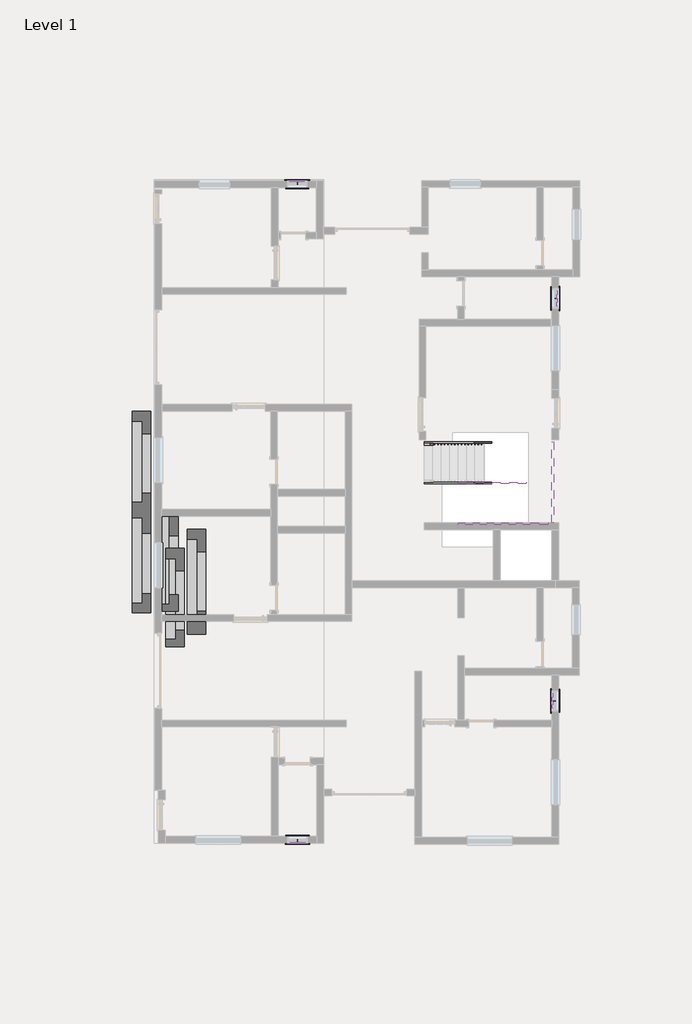
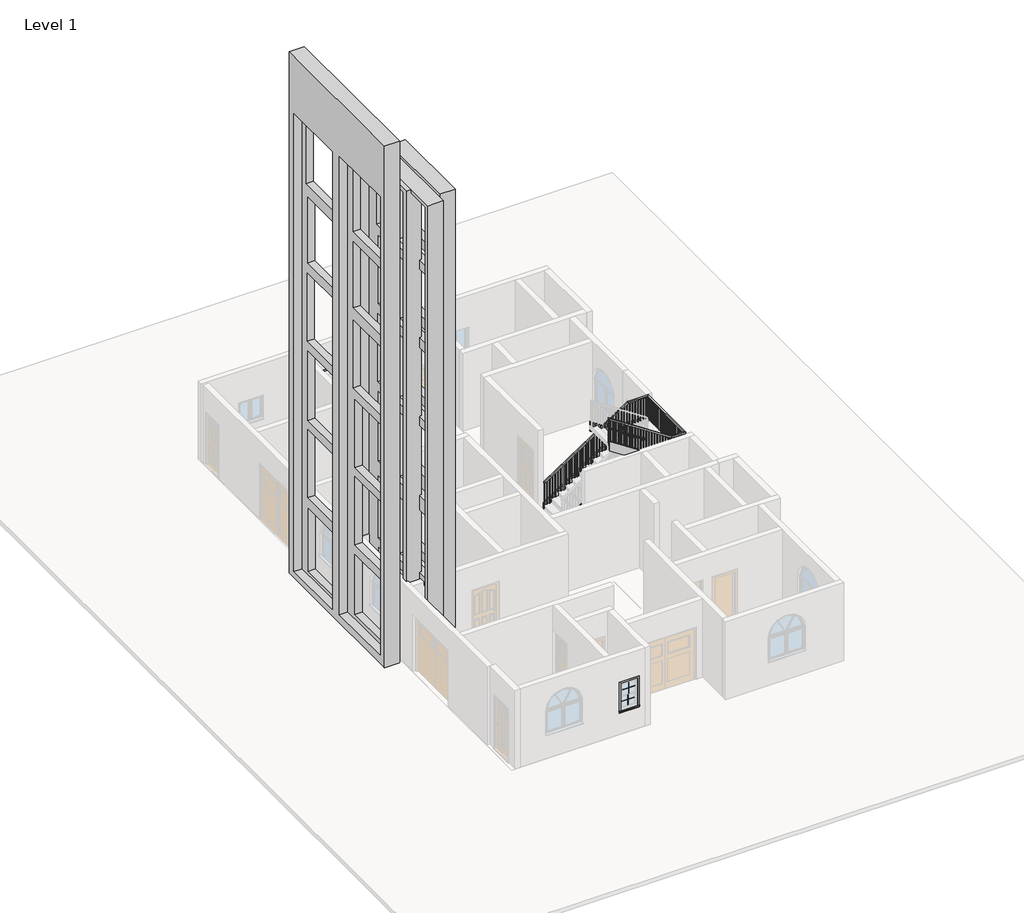
# One storey, part 4 of 4: 20 proxies, 5 members, 1 railing.
"""IFC4 building model written with IfcOpenShell, lengths in millimetres."""

from ifc_helpers import new_model, si_unit, frame, origin, place, context, project, spatial, polyline, outline, extrude, faceted_brep, transform, mapped, element, save
from components import generic_models_1_generic_models_1_14763b5c, generic_models_2_generic_models_1_16343201, generic_models_3_generic_models_1_639dc579, generic_models_4_generic_models_1_30fca322, muntin_pattern_2x2_muntin_pattern_2x2_eba6c5fb, trim_window_exterior_flat_with_sill_278e6a94, trim_window_interior_flat_picture_frame_e9fd5f45

model = new_model("IFC4")

# Units and contexts
model_context = context("Model", 3, world=origin())
ifc_project = project(units=[si_unit("LENGTHUNIT", "METRE", prefix="MILLI")], contexts=[model_context])

# Site, building, storey
site = spatial("IfcSite", under=ifc_project)
building = spatial("IfcBuilding", under=site)
storey = spatial("IfcBuildingStorey", under=building, Name="Level 1", Elevation=0.0)

# Proxies
placement = place(None, origin())
generic_models_1_generic_models_1_shape = generic_models_1_generic_models_1_14763b5c(model_context)
element("IfcBuildingElementProxy", 1, Name="Generic Models 1 : Generic Models 1", ObjectType="Generic Models 1 : Generic Models 1", at=placement, inside=storey, context=model_context, shape_type="MappedRepresentation", body=[
    mapped(generic_models_1_generic_models_1_shape, transform((0.0, 0.0, 0.0), x_axis=(1.0, 0.0, 0.0), y_axis=(0.0, 1.0, 0.0), z_axis=(0.0, 0.0, 1.0))),
])
generic_models_2_generic_models_1_shape = generic_models_2_generic_models_1_16343201(model_context)
element("IfcBuildingElementProxy", 2, Name="Generic Models 2 : Generic Models 1", ObjectType="Generic Models 2 : Generic Models 1", at=placement, inside=storey, context=model_context, shape_type="MappedRepresentation", body=[
    mapped(generic_models_2_generic_models_1_shape, transform((824.2499329, -3076.1426277, 0.0), x_axis=(1.0, 0.0, 0.0), y_axis=(0.0, 1.0, 0.0), z_axis=(0.0, 0.0, 1.0))),
])
generic_models_3_generic_models_1_shape = generic_models_3_generic_models_1_639dc579(model_context)
element("IfcBuildingElementProxy", 3, Name="Generic Models 3 : Generic Models 1", ObjectType="Generic Models 3 : Generic Models 1", at=placement, inside=storey, context=model_context, shape_type="MappedRepresentation", body=[
    mapped(generic_models_3_generic_models_1_shape, transform((1011.525957, -4144.962921, 0.0), x_axis=(1.0, 0.0, 0.0), y_axis=(0.0, 1.0, 0.0), z_axis=(0.0, 0.0, 1.0))),
])
generic_models_4_generic_models_1_shape = generic_models_4_generic_models_1_30fca322(model_context)
element("IfcBuildingElementProxy", 4, Name="Generic Models 4 : Generic Models 1", ObjectType="Generic Models 4 : Generic Models 1", at=placement, inside=storey, context=model_context, shape_type="MappedRepresentation", body=[
    mapped(generic_models_4_generic_models_1_shape, transform((1663.8480965, -3568.1337576, 0.0), x_axis=(1.0, 0.0, 0.0), y_axis=(0.0, 1.0, 0.0), z_axis=(0.0, 0.0, 1.0))),
])
muntin_pattern_2x2_muntin_pattern_2x2_shape = muntin_pattern_2x2_muntin_pattern_2x2_eba6c5fb(model_context)
element("IfcBuildingElementProxy", 5, Name="Muntin Pattern_2x2 : Muntin Pattern_2x2", ObjectType="Muntin Pattern_2x2 : Muntin Pattern_2x2", at=placement, inside=storey, context=model_context, shape_type="MappedRepresentation", body=[
    mapped(muntin_pattern_2x2_muntin_pattern_2x2_shape, transform((5828.2640963, 5846.2962251, 1470.025), x_axis=(0.0, -1.0, 0.0), y_axis=(1.0, 0.0, 0.0), z_axis=(0.0, 0.0, 1.0))),
])
element("IfcBuildingElementProxy", 6, Name="Muntin Pattern_2x2 : Muntin Pattern_2x2", ObjectType="Muntin Pattern_2x2 : Muntin Pattern_2x2", at=placement, inside=storey, context=model_context, shape_type="MappedRepresentation", body=[
    mapped(muntin_pattern_2x2_muntin_pattern_2x2_shape, transform((5783.8140963, 5846.2962251, 990.6), x_axis=(0.0, -1.0, 0.0), y_axis=(1.0, 0.0, 0.0), z_axis=(0.0, 0.0, 1.0))),
])
element("IfcBuildingElementProxy", 7, Name="Muntin Pattern_2x2 : Muntin Pattern_2x2", ObjectType="Muntin Pattern_2x2 : Muntin Pattern_2x2", at=placement, inside=storey, context=model_context, shape_type="MappedRepresentation", body=[
    mapped(muntin_pattern_2x2_muntin_pattern_2x2_shape, transform((5694.9140963, -6313.9537749, 1470.025), x_axis=(0.0, 1.0, 0.0), y_axis=(-1.0, 0.0, 0.0), z_axis=(0.0, 0.0, 1.0))),
])
element("IfcBuildingElementProxy", 8, Name="Muntin Pattern_2x2 : Muntin Pattern_2x2", ObjectType="Muntin Pattern_2x2 : Muntin Pattern_2x2", at=placement, inside=storey, context=model_context, shape_type="MappedRepresentation", body=[
    mapped(muntin_pattern_2x2_muntin_pattern_2x2_shape, transform((5739.3640963, -6313.9537749, 990.6), x_axis=(0.0, 1.0, 0.0), y_axis=(-1.0, 0.0, 0.0), z_axis=(0.0, 0.0, 1.0))),
])
element("IfcBuildingElementProxy", 9, Name="Muntin Pattern_2x2 : Muntin Pattern_2x2", ObjectType="Muntin Pattern_2x2 : Muntin Pattern_2x2", at=placement, inside=storey, context=model_context, shape_type="MappedRepresentation", body=[
    mapped(muntin_pattern_2x2_muntin_pattern_2x2_shape, transform((-2029.8609037, 9366.9277313, 1470.025), x_axis=(1.0, 0.0, 0.0), y_axis=(0.0, 1.0, 0.0), z_axis=(0.0, 0.0, 1.0))),
])
element("IfcBuildingElementProxy", 10, Name="Muntin Pattern_2x2 : Muntin Pattern_2x2", ObjectType="Muntin Pattern_2x2 : Muntin Pattern_2x2", at=placement, inside=storey, context=model_context, shape_type="MappedRepresentation", body=[
    mapped(muntin_pattern_2x2_muntin_pattern_2x2_shape, transform((-2029.8609037, 9322.4777313, 990.6), x_axis=(1.0, 0.0, 0.0), y_axis=(0.0, 1.0, 0.0), z_axis=(0.0, 0.0, 1.0))),
])
element("IfcBuildingElementProxy", 11, Name="Muntin Pattern_2x2 : Muntin Pattern_2x2", ObjectType="Muntin Pattern_2x2 : Muntin Pattern_2x2", at=placement, inside=storey, context=model_context, shape_type="MappedRepresentation", body=[
    mapped(muntin_pattern_2x2_muntin_pattern_2x2_shape, transform((-2023.5109037, -10577.9787749, 1470.025), x_axis=(-1.0, 0.0, 0.0), y_axis=(0.0, -1.0, 0.0), z_axis=(0.0, 0.0, 1.0))),
])
element("IfcBuildingElementProxy", 12, Name="Muntin Pattern_2x2 : Muntin Pattern_2x2", ObjectType="Muntin Pattern_2x2 : Muntin Pattern_2x2", at=placement, inside=storey, context=model_context, shape_type="MappedRepresentation", body=[
    mapped(muntin_pattern_2x2_muntin_pattern_2x2_shape, transform((-2023.5109037, -10533.5287749, 990.6), x_axis=(-1.0, 0.0, 0.0), y_axis=(0.0, -1.0, 0.0), z_axis=(0.0, 0.0, 1.0))),
])
trim_window_exterior_flat_with_sill_shape = trim_window_exterior_flat_with_sill_278e6a94(model_context)
element("IfcBuildingElementProxy", 13, Name="Trim-Window-Exterior-Flat : with Sill", ObjectType="Trim-Window-Exterior-Flat : with Sill", at=placement, inside=storey, context=model_context, shape_type="MappedRepresentation", body=[
    mapped(trim_window_exterior_flat_with_sill_shape, transform((5863.1890963, 5846.2962251, 1981.2), x_axis=(0.0, 1.0, 0.0), y_axis=(0.0, 0.0, 1.0), z_axis=(1.0, 0.0, 0.0))),
])
element("IfcBuildingElementProxy", 14, Name="Trim-Window-Exterior-Flat : with Sill", ObjectType="Trim-Window-Exterior-Flat : with Sill", at=placement, inside=storey, context=model_context, shape_type="MappedRepresentation", body=[
    mapped(trim_window_exterior_flat_with_sill_shape, transform((5659.9890963, -6313.9537749, 1981.2), x_axis=(0.0, -1.0, 0.0), y_axis=(0.0, 0.0, 1.0), z_axis=(-1.0, 0.0, 0.0))),
])
element("IfcBuildingElementProxy", 15, Name="Trim-Window-Exterior-Flat : with Sill", ObjectType="Trim-Window-Exterior-Flat : with Sill", at=placement, inside=storey, context=model_context, shape_type="MappedRepresentation", body=[
    mapped(trim_window_exterior_flat_with_sill_shape, transform((-2029.8609037, 9401.8527313, 1981.2), x_axis=(-1.0, 0.0, 0.0), y_axis=(0.0, 0.0, 1.0), z_axis=(0.0, 1.0, 0.0))),
])
element("IfcBuildingElementProxy", 16, Name="Trim-Window-Exterior-Flat : with Sill", ObjectType="Trim-Window-Exterior-Flat : with Sill", at=placement, inside=storey, context=model_context, shape_type="MappedRepresentation", body=[
    mapped(trim_window_exterior_flat_with_sill_shape, transform((-2023.5109037, -10612.9037749, 1981.2), x_axis=(1.0, 0.0, 0.0), y_axis=(0.0, 0.0, 1.0), z_axis=(0.0, -1.0, 0.0))),
])
trim_window_interior_flat_picture_frame_shape = trim_window_interior_flat_picture_frame_e9fd5f45(model_context)
element("IfcBuildingElementProxy", 17, Name="Trim-Window-Interior-Flat : Picture Frame", ObjectType="Trim-Window-Interior-Flat : Picture Frame", at=placement, inside=storey, context=model_context, shape_type="MappedRepresentation", body=[
    mapped(trim_window_interior_flat_picture_frame_shape, transform((5659.9890963, 5846.2962251, 1981.2), x_axis=(0.0, -1.0, 0.0), y_axis=(0.0, 0.0, 1.0), z_axis=(-1.0, 0.0, 0.0))),
])
element("IfcBuildingElementProxy", 18, Name="Trim-Window-Interior-Flat : Picture Frame", ObjectType="Trim-Window-Interior-Flat : Picture Frame", at=placement, inside=storey, context=model_context, shape_type="MappedRepresentation", body=[
    mapped(trim_window_interior_flat_picture_frame_shape, transform((5863.1890963, -6313.9537749, 1981.2), x_axis=(0.0, 1.0, 0.0), y_axis=(0.0, 0.0, 1.0), z_axis=(1.0, 0.0, 0.0))),
])
element("IfcBuildingElementProxy", 19, Name="Trim-Window-Interior-Flat : Picture Frame", ObjectType="Trim-Window-Interior-Flat : Picture Frame", at=placement, inside=storey, context=model_context, shape_type="MappedRepresentation", body=[
    mapped(trim_window_interior_flat_picture_frame_shape, transform((-2029.8609037, 9198.6527313, 1981.2), x_axis=(1.0, 0.0, 0.0), y_axis=(0.0, 0.0, 1.0), z_axis=(0.0, -1.0, 0.0))),
])
element("IfcBuildingElementProxy", 20, Name="Trim-Window-Interior-Flat : Picture Frame", ObjectType="Trim-Window-Interior-Flat : Picture Frame", at=placement, inside=storey, context=model_context, shape_type="MappedRepresentation", body=[
    mapped(trim_window_interior_flat_picture_frame_shape, transform((-2023.5109037, -10409.7037749, 1981.2), x_axis=(-1.0, 0.0, 0.0), y_axis=(0.0, 0.0, 1.0), z_axis=(0.0, 1.0, 0.0))),
])

# Members
element("IfcMember", 21, ObjectType="Stringer - 2\" Width", at=placement, inside=storey, context=model_context, shape_type="SweptSolid", body=[
    extrude(outline(polyline([(218.8021702, 1811.8890963), (0.0, 1811.8890963), (0.0, 2033.570289), (2277.5333333, 5475.7230993), (2277.5333333, 4923.3549769), (218.8021702, 1811.8890963)])), frame((0.0, 1464.7962251, 0.0), z_axis=(0.0, 1.0, 0.0), x_axis=(0.0, 0.0, 1.0)), (0.0, 0.0, 1.0), 50.8),
])
element("IfcMember", 22, ObjectType="Stringer - 2\" Width", at=placement, inside=storey, context=model_context, shape_type="SweptSolid", body=[
    extrude(outline(polyline([(5659.9890963, 1515.5962251), (5710.7890963, 1515.5962251), (5710.7890963, -935.5037749), (5659.9890963, -935.5037749), (5659.9890963, 1515.5962251)])), frame((0.0, 0.0, 1972.7333333), z_axis=(0.0, 0.0, 1.0), x_axis=(1.0, 0.0, 0.0)), (0.0, 0.0, 1.0), 304.8),
])
element("IfcMember", 23, ObjectType="Stringer - 2\" Width", at=placement, inside=storey, context=model_context, shape_type="SweptSolid", body=[
    extrude(outline(polyline([(1972.7333333, 5557.7517847), (3771.2542006, 2827.8890963), (3406.2494122, 2827.8890963), (1972.7333333, 5003.7337741), (1972.7333333, 5557.7517847)])), frame((0.0, -986.3037749, 0.0), z_axis=(0.0, 1.0, 0.0), x_axis=(0.0, 0.0, 1.0)), (0.0, 0.0, 1.0), 50.8),
])
element("IfcMember", 24, ObjectType="Stringer - 2\" Width", at=placement, inside=storey, context=model_context, shape_type="SweptSolid", body=[
    extrude(outline(polyline([(218.8021702, 1811.8890963), (0.0, 1811.8890963), (0.0, 2033.570289), (1850.4384087, 4830.2326586), (2215.9180606, 4830.2326586), (218.8021702, 1811.8890963)])), frame((0.0, 245.5962251, 0.0), z_axis=(0.0, 1.0, 0.0), x_axis=(0.0, 0.0, 1.0)), (0.0, 0.0, 1.0), 50.8),
])
element("IfcMember", 25, ObjectType="Stringer - 2\" Width", at=placement, inside=storey, context=model_context, shape_type="SweptSolid", body=[
    extrude(outline(polyline([(2053.5727534, 4881.0326586), (2418.5775418, 4881.0326586), (3771.2542006, 2827.8890963), (3406.2494122, 2827.8890963), (2053.5727534, 4881.0326586)])), frame((0.0, 245.5962251, 0.0), z_axis=(0.0, 1.0, 0.0), x_axis=(0.0, 0.0, 1.0)), (0.0, 0.0, 1.0), 50.8),
])

# Railing
element("IfcRailing", 26, ObjectType="Handrail - Rectangular", at=placement, inside=storey, context=model_context, shape_type="SolidModel", body=[
    faceted_brep([(1811.8890963, 1464.7962251, 1083.7333333), (1811.8890963, 1464.7962251, 1022.8084396), (1811.8890963, 1413.9962251, 1022.8084396), (1811.8890963, 1413.9962251, 1083.7333333), (4881.0326586, 1464.7962251, 3115.7333333), (4896.3253517, 1464.7962251, 3064.9333333), (4896.3253517, 1413.9962251, 3064.9333333), (4881.0326586, 1413.9962251, 3115.7333333), (5659.9890963, 1464.7962251, 3115.7333333), (5659.9890963, 1464.7962251, 3064.9333333), (5609.1890963, 1413.9962251, 3064.9333333), (5609.1890963, 1413.9962251, 3115.7333333), (5659.9890963, -935.5037749, 3115.7333333), (5659.9890963, -935.5037749, 3064.9333333), (5609.1890963, -884.7037749, 3064.9333333), (5609.1890963, -884.7037749, 3115.7333333), (5137.6756039, -935.5037749, 3115.7333333), (5122.4267175, -935.5037749, 3064.9333333), (5122.4267175, -884.7037749, 3064.9333333), (5137.6756039, -884.7037749, 3115.7333333), (2827.8890963, -935.5037749, 4639.7333333), (2827.8890963, -884.7037749, 4639.7333333), (2827.8890963, -884.7037749, 4578.8720992), (2827.8890963, -935.5037749, 4578.8720992)], [[[0, 1, 2, 3]], [[1, 0, 4, 5]], [[2, 1, 5, 6]], [[3, 2, 6, 7]], [[0, 3, 7, 4]], [[5, 4, 8, 9]], [[6, 5, 9, 10]], [[7, 6, 10, 11]], [[4, 7, 11, 8]], [[9, 8, 12, 13]], [[10, 9, 13, 14]], [[11, 10, 14, 15]], [[8, 11, 15, 12]], [[13, 12, 16, 17]], [[14, 13, 17, 18]], [[15, 14, 18, 19]], [[12, 15, 19, 16]], [[20, 21, 22, 23]], [[17, 16, 20, 23]], [[18, 17, 23, 22]], [[19, 18, 22, 21]], [[16, 19, 21, 20]]]),
    extrude(outline(polyline([(4543.3154863, 2881.8640963), (3556.0, 2881.8640963), (3556.0, 2900.9140963), (4530.7029775, 2900.9140963), (4543.3154863, 2881.8640963)])), frame((0.0, -919.6287749, 0.0), z_axis=(0.0, 1.0, 0.0), x_axis=(0.0, 0.0, 1.0)), (0.0, 0.0, 1.0), 19.05),
    extrude(outline(polyline([(4476.2235214, 2983.4640963), (3556.0, 2983.4640963), (3556.0, 3002.5140963), (4463.6543078, 3002.5140963), (4476.2235214, 2983.4640963)])), frame((0.0, -919.6287749, 0.0), z_axis=(0.0, 1.0, 0.0), x_axis=(0.0, 0.0, 1.0)), (0.0, 0.0, 1.0), 19.05),
    extrude(outline(polyline([(4409.1877155, 3085.0640963), (3386.6666667, 3085.0640963), (3386.6666667, 3104.1140963), (4396.6185019, 3104.1140963), (4409.1877155, 3085.0640963)])), frame((0.0, -919.6287749, 0.0), z_axis=(0.0, 1.0, 0.0), x_axis=(0.0, 0.0, 1.0)), (0.0, 0.0, 1.0), 19.05),
    extrude(outline(polyline([(4342.1519096, 3186.6640963), (3386.6666667, 3186.6640963), (3386.6666667, 3205.7140963), (4329.582696, 3205.7140963), (4342.1519096, 3186.6640963)])), frame((0.0, -919.6287749, 0.0), z_axis=(0.0, 1.0, 0.0), x_axis=(0.0, 0.0, 1.0)), (0.0, 0.0, 1.0), 19.05),
    extrude(outline(polyline([(4275.1161037, 3288.2640963), (3386.6666667, 3288.2640963), (3386.6666667, 3307.3140963), (4262.5468901, 3307.3140963), (4275.1161037, 3288.2640963)])), frame((0.0, -919.6287749, 0.0), z_axis=(0.0, 1.0, 0.0), x_axis=(0.0, 0.0, 1.0)), (0.0, 0.0, 1.0), 19.05),
    extrude(outline(polyline([(4208.0802978, 3389.8640963), (3217.3333333, 3389.8640963), (3217.3333333, 3408.9140963), (4195.5110842, 3408.9140963), (4208.0802978, 3389.8640963)])), frame((0.0, -919.6287749, 0.0), z_axis=(0.0, 1.0, 0.0), x_axis=(0.0, 0.0, 1.0)), (0.0, 0.0, 1.0), 19.05),
    extrude(outline(polyline([(4141.0444919, 3491.4640963), (3217.3333333, 3491.4640963), (3217.3333333, 3510.5140963), (4128.4752783, 3510.5140963), (4141.0444919, 3491.4640963)])), frame((0.0, -919.6287749, 0.0), z_axis=(0.0, 1.0, 0.0), x_axis=(0.0, 0.0, 1.0)), (0.0, 0.0, 1.0), 19.05),
    extrude(outline(polyline([(4074.008686, 3593.0640963), (3048.0, 3593.0640963), (3048.0, 3612.1140963), (4061.4394724, 3612.1140963), (4074.008686, 3593.0640963)])), frame((0.0, -919.6287749, 0.0), z_axis=(0.0, 1.0, 0.0), x_axis=(0.0, 0.0, 1.0)), (0.0, 0.0, 1.0), 19.05),
    extrude(outline(polyline([(4006.9728801, 3694.6640963), (3048.0, 3694.6640963), (3048.0, 3713.7140963), (3994.4036665, 3713.7140963), (4006.9728801, 3694.6640963)])), frame((0.0, -919.6287749, 0.0), z_axis=(0.0, 1.0, 0.0), x_axis=(0.0, 0.0, 1.0)), (0.0, 0.0, 1.0), 19.05),
    extrude(outline(polyline([(3939.9370742, 3796.2640963), (3048.0, 3796.2640963), (3048.0, 3815.3140963), (3927.3678606, 3815.3140963), (3939.9370742, 3796.2640963)])), frame((0.0, -919.6287749, 0.0), z_axis=(0.0, 1.0, 0.0), x_axis=(0.0, 0.0, 1.0)), (0.0, 0.0, 1.0), 19.05),
    extrude(outline(polyline([(3872.9814538, 3897.8640963), (2878.6666667, 3897.8640963), (2878.6666667, 3916.9140963), (3860.3689451, 3916.9140963), (3872.9814538, 3897.8640963)])), frame((0.0, -919.6287749, 0.0), z_axis=(0.0, 1.0, 0.0), x_axis=(0.0, 0.0, 1.0)), (0.0, 0.0, 1.0), 19.05),
    extrude(outline(polyline([(3805.8654624, 3999.4640963), (2878.6666667, 3999.4640963), (2878.6666667, 4018.5140963), (3793.2962488, 4018.5140963), (3805.8654624, 3999.4640963)])), frame((0.0, -919.6287749, 0.0), z_axis=(0.0, 1.0, 0.0), x_axis=(0.0, 0.0, 1.0)), (0.0, 0.0, 1.0), 19.05),
    extrude(outline(polyline([(3738.8296565, 4101.0640963), (2709.3333333, 4101.0640963), (2709.3333333, 4120.1140963), (3726.2604429, 4120.1140963), (3738.8296565, 4101.0640963)])), frame((0.0, -919.6287749, 0.0), z_axis=(0.0, 1.0, 0.0), x_axis=(0.0, 0.0, 1.0)), (0.0, 0.0, 1.0), 19.05),
    extrude(outline(polyline([(3671.7938506, 4202.6640963), (2709.3333333, 4202.6640963), (2709.3333333, 4221.7140963), (3659.224637, 4221.7140963), (3671.7938506, 4202.6640963)])), frame((0.0, -919.6287749, 0.0), z_axis=(0.0, 1.0, 0.0), x_axis=(0.0, 0.0, 1.0)), (0.0, 0.0, 1.0), 19.05),
    extrude(outline(polyline([(3604.7580447, 4304.2640963), (2709.3333333, 4304.2640963), (2709.3333333, 4323.3140963), (3592.1888311, 4323.3140963), (3604.7580447, 4304.2640963)])), frame((0.0, -919.6287749, 0.0), z_axis=(0.0, 1.0, 0.0), x_axis=(0.0, 0.0, 1.0)), (0.0, 0.0, 1.0), 19.05),
    extrude(outline(polyline([(3537.7222388, 4405.8640963), (2540.0, 4405.8640963), (2540.0, 4424.9140963), (3525.1530252, 4424.9140963), (3537.7222388, 4405.8640963)])), frame((0.0, -919.6287749, 0.0), z_axis=(0.0, 1.0, 0.0), x_axis=(0.0, 0.0, 1.0)), (0.0, 0.0, 1.0), 19.05),
    extrude(outline(polyline([(3470.6864329, 4507.4640963), (2540.0, 4507.4640963), (2540.0, 4526.5140963), (3458.1172193, 4526.5140963), (3470.6864329, 4507.4640963)])), frame((0.0, -919.6287749, 0.0), z_axis=(0.0, 1.0, 0.0), x_axis=(0.0, 0.0, 1.0)), (0.0, 0.0, 1.0), 19.05),
    extrude(outline(polyline([(3403.650627, 4609.0640963), (2370.6666667, 4609.0640963), (2370.6666667, 4628.1140963), (3391.0814134, 4628.1140963), (3403.650627, 4609.0640963)])), frame((0.0, -919.6287749, 0.0), z_axis=(0.0, 1.0, 0.0), x_axis=(0.0, 0.0, 1.0)), (0.0, 0.0, 1.0), 19.05),
    extrude(outline(polyline([(3336.6148211, 4710.6640963), (2370.6666667, 4710.6640963), (2370.6666667, 4729.7140963), (3324.0456075, 4729.7140963), (3336.6148211, 4710.6640963)])), frame((0.0, -919.6287749, 0.0), z_axis=(0.0, 1.0, 0.0), x_axis=(0.0, 0.0, 1.0)), (0.0, 0.0, 1.0), 19.05),
    extrude(outline(polyline([(3269.5790152, 4812.2640963), (2370.6666667, 4812.2640963), (2370.6666667, 4831.3140963), (3257.0098016, 4831.3140963), (3269.5790152, 4812.2640963)])), frame((0.0, -919.6287749, 0.0), z_axis=(0.0, 1.0, 0.0), x_axis=(0.0, 0.0, 1.0)), (0.0, 0.0, 1.0), 19.05),
    extrude(outline(polyline([(3202.5432093, 4913.8640963), (2201.3333333, 4913.8640963), (2201.3333333, 4932.9140963), (3189.9739957, 4932.9140963), (3202.5432093, 4913.8640963)])), frame((0.0, -919.6287749, 0.0), z_axis=(0.0, 1.0, 0.0), x_axis=(0.0, 0.0, 1.0)), (0.0, 0.0, 1.0), 19.05),
    extrude(outline(polyline([(3135.5074034, 5015.4640963), (2201.3333333, 5015.4640963), (2201.3333333, 5034.5140963), (3122.9381898, 5034.5140963), (3135.5074034, 5015.4640963)])), frame((0.0, -919.6287749, 0.0), z_axis=(0.0, 1.0, 0.0), x_axis=(0.0, 0.0, 1.0)), (0.0, 0.0, 1.0), 19.05),
    extrude(outline(polyline([(3068.4715975, 5117.0640963), (2201.3333333, 5117.0640963), (2201.3333333, 5136.1140963), (3055.9023839, 5136.1140963), (3068.4715975, 5117.0640963)])), frame((0.0, -919.6287749, 0.0), z_axis=(0.0, 1.0, 0.0), x_axis=(0.0, 0.0, 1.0)), (0.0, 0.0, 1.0), 19.05),
    extrude(outline(polyline([(5237.7140963, -919.6287749), (5218.6640963, -919.6287749), (5218.6640963, -900.5787749), (5237.7140963, -900.5787749), (5237.7140963, -919.6287749)])), frame((0.0, 0.0, 2201.3333333), z_axis=(0.0, 0.0, 1.0), x_axis=(1.0, 0.0, 0.0)), (0.0, 0.0, 1.0), 863.6),
    extrude(outline(polyline([(5339.3140963, -919.6287749), (5320.2640963, -919.6287749), (5320.2640963, -900.5787749), (5339.3140963, -900.5787749), (5339.3140963, -919.6287749)])), frame((0.0, 0.0, 2201.3333333), z_axis=(0.0, 0.0, 1.0), x_axis=(1.0, 0.0, 0.0)), (0.0, 0.0, 1.0), 863.6),
    extrude(outline(polyline([(5440.9140963, -919.6287749), (5421.8640963, -919.6287749), (5421.8640963, -900.5787749), (5440.9140963, -900.5787749), (5440.9140963, -919.6287749)])), frame((0.0, 0.0, 2201.3333333), z_axis=(0.0, 0.0, 1.0), x_axis=(1.0, 0.0, 0.0)), (0.0, 0.0, 1.0), 863.6),
    extrude(outline(polyline([(5542.5140963, -919.6287749), (5523.4640963, -919.6287749), (5523.4640963, -900.5787749), (5542.5140963, -900.5787749), (5542.5140963, -919.6287749)])), frame((0.0, 0.0, 2201.3333333), z_axis=(0.0, 0.0, 1.0), x_axis=(1.0, 0.0, 0.0)), (0.0, 0.0, 1.0), 863.6),
    extrude(outline(polyline([(5644.1140963, -887.8787749), (5644.1140963, -906.9287749), (5625.0640963, -906.9287749), (5625.0640963, -887.8787749), (5644.1140963, -887.8787749)])), frame((0.0, 0.0, 2201.3333333), z_axis=(0.0, 0.0, 1.0), x_axis=(1.0, 0.0, 0.0)), (0.0, 0.0, 1.0), 863.6),
    extrude(outline(polyline([(5644.1140963, -786.2787749), (5644.1140963, -805.3287749), (5625.0640963, -805.3287749), (5625.0640963, -786.2787749), (5644.1140963, -786.2787749)])), frame((0.0, 0.0, 2201.3333333), z_axis=(0.0, 0.0, 1.0), x_axis=(1.0, 0.0, 0.0)), (0.0, 0.0, 1.0), 863.6),
    extrude(outline(polyline([(5644.1140963, -684.6787749), (5644.1140963, -703.7287749), (5625.0640963, -703.7287749), (5625.0640963, -684.6787749), (5644.1140963, -684.6787749)])), frame((0.0, 0.0, 2201.3333333), z_axis=(0.0, 0.0, 1.0), x_axis=(1.0, 0.0, 0.0)), (0.0, 0.0, 1.0), 863.6),
    extrude(outline(polyline([(5644.1140963, -583.0787749), (5644.1140963, -602.1287749), (5625.0640963, -602.1287749), (5625.0640963, -583.0787749), (5644.1140963, -583.0787749)])), frame((0.0, 0.0, 2201.3333333), z_axis=(0.0, 0.0, 1.0), x_axis=(1.0, 0.0, 0.0)), (0.0, 0.0, 1.0), 863.6),
    extrude(outline(polyline([(5644.1140963, -481.4787749), (5644.1140963, -500.5287749), (5625.0640963, -500.5287749), (5625.0640963, -481.4787749), (5644.1140963, -481.4787749)])), frame((0.0, 0.0, 2201.3333333), z_axis=(0.0, 0.0, 1.0), x_axis=(1.0, 0.0, 0.0)), (0.0, 0.0, 1.0), 863.6),
    extrude(outline(polyline([(5644.1140963, -379.8787749), (5644.1140963, -398.9287749), (5625.0640963, -398.9287749), (5625.0640963, -379.8787749), (5644.1140963, -379.8787749)])), frame((0.0, 0.0, 2201.3333333), z_axis=(0.0, 0.0, 1.0), x_axis=(1.0, 0.0, 0.0)), (0.0, 0.0, 1.0), 863.6),
    extrude(outline(polyline([(5644.1140963, -278.2787749), (5644.1140963, -297.3287749), (5625.0640963, -297.3287749), (5625.0640963, -278.2787749), (5644.1140963, -278.2787749)])), frame((0.0, 0.0, 2201.3333333), z_axis=(0.0, 0.0, 1.0), x_axis=(1.0, 0.0, 0.0)), (0.0, 0.0, 1.0), 863.6),
    extrude(outline(polyline([(5644.1140963, -176.6787749), (5644.1140963, -195.7287749), (5625.0640963, -195.7287749), (5625.0640963, -176.6787749), (5644.1140963, -176.6787749)])), frame((0.0, 0.0, 2201.3333333), z_axis=(0.0, 0.0, 1.0), x_axis=(1.0, 0.0, 0.0)), (0.0, 0.0, 1.0), 863.6),
    extrude(outline(polyline([(5644.1140963, -75.0787749), (5644.1140963, -94.1287749), (5625.0640963, -94.1287749), (5625.0640963, -75.0787749), (5644.1140963, -75.0787749)])), frame((0.0, 0.0, 2201.3333333), z_axis=(0.0, 0.0, 1.0), x_axis=(1.0, 0.0, 0.0)), (0.0, 0.0, 1.0), 863.6),
    extrude(outline(polyline([(5644.1140963, 26.5212251), (5644.1140963, 7.4712251), (5625.0640963, 7.4712251), (5625.0640963, 26.5212251), (5644.1140963, 26.5212251)])), frame((0.0, 0.0, 2201.3333333), z_axis=(0.0, 0.0, 1.0), x_axis=(1.0, 0.0, 0.0)), (0.0, 0.0, 1.0), 863.6),
    extrude(outline(polyline([(5644.1140963, 128.1212251), (5644.1140963, 109.0712251), (5625.0640963, 109.0712251), (5625.0640963, 128.1212251), (5644.1140963, 128.1212251)])), frame((0.0, 0.0, 2201.3333333), z_axis=(0.0, 0.0, 1.0), x_axis=(1.0, 0.0, 0.0)), (0.0, 0.0, 1.0), 863.6),
    extrude(outline(polyline([(5644.1140963, 229.7212251), (5644.1140963, 210.6712251), (5625.0640963, 210.6712251), (5625.0640963, 229.7212251), (5644.1140963, 229.7212251)])), frame((0.0, 0.0, 2201.3333333), z_axis=(0.0, 0.0, 1.0), x_axis=(1.0, 0.0, 0.0)), (0.0, 0.0, 1.0), 863.6),
    extrude(outline(polyline([(5644.1140963, 331.3212251), (5644.1140963, 312.2712251), (5625.0640963, 312.2712251), (5625.0640963, 331.3212251), (5644.1140963, 331.3212251)])), frame((0.0, 0.0, 2201.3333333), z_axis=(0.0, 0.0, 1.0), x_axis=(1.0, 0.0, 0.0)), (0.0, 0.0, 1.0), 863.6),
    extrude(outline(polyline([(5644.1140963, 432.9212251), (5644.1140963, 413.8712251), (5625.0640963, 413.8712251), (5625.0640963, 432.9212251), (5644.1140963, 432.9212251)])), frame((0.0, 0.0, 2201.3333333), z_axis=(0.0, 0.0, 1.0), x_axis=(1.0, 0.0, 0.0)), (0.0, 0.0, 1.0), 863.6),
    extrude(outline(polyline([(5644.1140963, 534.5212251), (5644.1140963, 515.4712251), (5625.0640963, 515.4712251), (5625.0640963, 534.5212251), (5644.1140963, 534.5212251)])), frame((0.0, 0.0, 2201.3333333), z_axis=(0.0, 0.0, 1.0), x_axis=(1.0, 0.0, 0.0)), (0.0, 0.0, 1.0), 863.6),
    extrude(outline(polyline([(5644.1140963, 636.1212251), (5644.1140963, 617.0712251), (5625.0640963, 617.0712251), (5625.0640963, 636.1212251), (5644.1140963, 636.1212251)])), frame((0.0, 0.0, 2201.3333333), z_axis=(0.0, 0.0, 1.0), x_axis=(1.0, 0.0, 0.0)), (0.0, 0.0, 1.0), 863.6),
    extrude(outline(polyline([(5644.1140963, 737.7212251), (5644.1140963, 718.6712251), (5625.0640963, 718.6712251), (5625.0640963, 737.7212251), (5644.1140963, 737.7212251)])), frame((0.0, 0.0, 2201.3333333), z_axis=(0.0, 0.0, 1.0), x_axis=(1.0, 0.0, 0.0)), (0.0, 0.0, 1.0), 863.6),
    extrude(outline(polyline([(5644.1140963, 839.3212251), (5644.1140963, 820.2712251), (5625.0640963, 820.2712251), (5625.0640963, 839.3212251), (5644.1140963, 839.3212251)])), frame((0.0, 0.0, 2201.3333333), z_axis=(0.0, 0.0, 1.0), x_axis=(1.0, 0.0, 0.0)), (0.0, 0.0, 1.0), 863.6),
    extrude(outline(polyline([(5644.1140963, 940.9212251), (5644.1140963, 921.8712251), (5625.0640963, 921.8712251), (5625.0640963, 940.9212251), (5644.1140963, 940.9212251)])), frame((0.0, 0.0, 2201.3333333), z_axis=(0.0, 0.0, 1.0), x_axis=(1.0, 0.0, 0.0)), (0.0, 0.0, 1.0), 863.6),
    extrude(outline(polyline([(5644.1140963, 1042.5212251), (5644.1140963, 1023.4712251), (5625.0640963, 1023.4712251), (5625.0640963, 1042.5212251), (5644.1140963, 1042.5212251)])), frame((0.0, 0.0, 2201.3333333), z_axis=(0.0, 0.0, 1.0), x_axis=(1.0, 0.0, 0.0)), (0.0, 0.0, 1.0), 863.6),
    extrude(outline(polyline([(5644.1140963, 1144.1212251), (5644.1140963, 1125.0712251), (5625.0640963, 1125.0712251), (5625.0640963, 1144.1212251), (5644.1140963, 1144.1212251)])), frame((0.0, 0.0, 2201.3333333), z_axis=(0.0, 0.0, 1.0), x_axis=(1.0, 0.0, 0.0)), (0.0, 0.0, 1.0), 863.6),
    extrude(outline(polyline([(5644.1140963, 1245.7212251), (5644.1140963, 1226.6712251), (5625.0640963, 1226.6712251), (5625.0640963, 1245.7212251), (5644.1140963, 1245.7212251)])), frame((0.0, 0.0, 2201.3333333), z_axis=(0.0, 0.0, 1.0), x_axis=(1.0, 0.0, 0.0)), (0.0, 0.0, 1.0), 863.6),
    extrude(outline(polyline([(5644.1140963, 1347.3212251), (5644.1140963, 1328.2712251), (5625.0640963, 1328.2712251), (5625.0640963, 1347.3212251), (5644.1140963, 1347.3212251)])), frame((0.0, 0.0, 2201.3333333), z_axis=(0.0, 0.0, 1.0), x_axis=(1.0, 0.0, 0.0)), (0.0, 0.0, 1.0), 863.6),
    extrude(outline(polyline([(5561.5640963, 1448.9212251), (5580.6140963, 1448.9212251), (5580.6140963, 1429.8712251), (5561.5640963, 1429.8712251), (5561.5640963, 1448.9212251)])), frame((0.0, 0.0, 2201.3333333), z_axis=(0.0, 0.0, 1.0), x_axis=(1.0, 0.0, 0.0)), (0.0, 0.0, 1.0), 863.6),
    extrude(outline(polyline([(5459.9640963, 1448.9212251), (5479.0140963, 1448.9212251), (5479.0140963, 1429.8712251), (5459.9640963, 1429.8712251), (5459.9640963, 1448.9212251)])), frame((0.0, 0.0, 2201.3333333), z_axis=(0.0, 0.0, 1.0), x_axis=(1.0, 0.0, 0.0)), (0.0, 0.0, 1.0), 863.6),
    extrude(outline(polyline([(5358.3640963, 1448.9212251), (5377.4140963, 1448.9212251), (5377.4140963, 1429.8712251), (5358.3640963, 1429.8712251), (5358.3640963, 1448.9212251)])), frame((0.0, 0.0, 2201.3333333), z_axis=(0.0, 0.0, 1.0), x_axis=(1.0, 0.0, 0.0)), (0.0, 0.0, 1.0), 863.6),
    extrude(outline(polyline([(5256.7640963, 1448.9212251), (5275.8140963, 1448.9212251), (5275.8140963, 1429.8712251), (5256.7640963, 1429.8712251), (5256.7640963, 1448.9212251)])), frame((0.0, 0.0, 2201.3333333), z_axis=(0.0, 0.0, 1.0), x_axis=(1.0, 0.0, 0.0)), (0.0, 0.0, 1.0), 863.6),
    extrude(outline(polyline([(5155.1640963, 1448.9212251), (5174.2140963, 1448.9212251), (5174.2140963, 1429.8712251), (5155.1640963, 1429.8712251), (5155.1640963, 1448.9212251)])), frame((0.0, 0.0, 2201.3333333), z_axis=(0.0, 0.0, 1.0), x_axis=(1.0, 0.0, 0.0)), (0.0, 0.0, 1.0), 863.6),
    extrude(outline(polyline([(5053.5640963, 1448.9212251), (5072.6140963, 1448.9212251), (5072.6140963, 1429.8712251), (5053.5640963, 1429.8712251), (5053.5640963, 1448.9212251)])), frame((0.0, 0.0, 2201.3333333), z_axis=(0.0, 0.0, 1.0), x_axis=(1.0, 0.0, 0.0)), (0.0, 0.0, 1.0), 863.6),
    extrude(outline(polyline([(4951.9640963, 1448.9212251), (4971.0140963, 1448.9212251), (4971.0140963, 1429.8712251), (4951.9640963, 1429.8712251), (4951.9640963, 1448.9212251)])), frame((0.0, 0.0, 2201.3333333), z_axis=(0.0, 0.0, 1.0), x_axis=(1.0, 0.0, 0.0)), (0.0, 0.0, 1.0), 863.6),
    extrude(outline(polyline([(3034.5035834, 4850.3640963), (2032.0, 4850.3640963), (2032.0, 4869.4140963), (3047.1160921, 4869.4140963), (3034.5035834, 4850.3640963)])), frame((0.0, 1429.8712251, 0.0), z_axis=(0.0, 1.0, 0.0), x_axis=(0.0, 0.0, 1.0)), (0.0, 0.0, 1.0), 19.05),
    extrude(outline(polyline([(2967.2368701, 4748.7640963), (2032.0, 4748.7640963), (2032.0, 4767.8140963), (2979.8493789, 4767.8140963), (2967.2368701, 4748.7640963)])), frame((0.0, 1429.8712251, 0.0), z_axis=(0.0, 1.0, 0.0), x_axis=(0.0, 0.0, 1.0)), (0.0, 0.0, 1.0), 19.05),
    extrude(outline(polyline([(2899.9701569, 4647.1640963), (2032.0, 4647.1640963), (2032.0, 4666.2140963), (2912.5826656, 4666.2140963), (2899.9701569, 4647.1640963)])), frame((0.0, 1429.8712251, 0.0), z_axis=(0.0, 1.0, 0.0), x_axis=(0.0, 0.0, 1.0)), (0.0, 0.0, 1.0), 19.05),
    extrude(outline(polyline([(2832.7034436, 4545.5640963), (1862.6666667, 4545.5640963), (1862.6666667, 4564.6140963), (2845.3159523, 4564.6140963), (2832.7034436, 4545.5640963)])), frame((0.0, 1429.8712251, 0.0), z_axis=(0.0, 1.0, 0.0), x_axis=(0.0, 0.0, 1.0)), (0.0, 0.0, 1.0), 19.05),
    extrude(outline(polyline([(2765.4367303, 4443.9640963), (1862.6666667, 4443.9640963), (1862.6666667, 4463.0140963), (2778.049239, 4463.0140963), (2765.4367303, 4443.9640963)])), frame((0.0, 1429.8712251, 0.0), z_axis=(0.0, 1.0, 0.0), x_axis=(0.0, 0.0, 1.0)), (0.0, 0.0, 1.0), 19.05),
    extrude(outline(polyline([(2698.170017, 4342.3640963), (1862.6666667, 4342.3640963), (1862.6666667, 4361.4140963), (2710.7825258, 4361.4140963), (2698.170017, 4342.3640963)])), frame((0.0, 1429.8712251, 0.0), z_axis=(0.0, 1.0, 0.0), x_axis=(0.0, 0.0, 1.0)), (0.0, 0.0, 1.0), 19.05),
    extrude(outline(polyline([(2630.9033038, 4240.7640963), (1693.3333333, 4240.7640963), (1693.3333333, 4259.8140963), (2643.5158125, 4259.8140963), (2630.9033038, 4240.7640963)])), frame((0.0, 1429.8712251, 0.0), z_axis=(0.0, 1.0, 0.0), x_axis=(0.0, 0.0, 1.0)), (0.0, 0.0, 1.0), 19.05),
    extrude(outline(polyline([(2563.6365905, 4139.1640963), (1693.3333333, 4139.1640963), (1693.3333333, 4158.2140963), (2576.2490992, 4158.2140963), (2563.6365905, 4139.1640963)])), frame((0.0, 1429.8712251, 0.0), z_axis=(0.0, 1.0, 0.0), x_axis=(0.0, 0.0, 1.0)), (0.0, 0.0, 1.0), 19.05),
    extrude(outline(polyline([(2496.3698772, 4037.5640963), (1524.0, 4037.5640963), (1524.0, 4056.6140963), (2508.982386, 4056.6140963), (2496.3698772, 4037.5640963)])), frame((0.0, 1429.8712251, 0.0), z_axis=(0.0, 1.0, 0.0), x_axis=(0.0, 0.0, 1.0)), (0.0, 0.0, 1.0), 19.05),
    extrude(outline(polyline([(2429.1031639, 3935.9640963), (1524.0, 3935.9640963), (1524.0, 3955.0140963), (2441.7156727, 3955.0140963), (2429.1031639, 3935.9640963)])), frame((0.0, 1429.8712251, 0.0), z_axis=(0.0, 1.0, 0.0), x_axis=(0.0, 0.0, 1.0)), (0.0, 0.0, 1.0), 19.05),
    extrude(outline(polyline([(2361.8364507, 3834.3640963), (1524.0, 3834.3640963), (1524.0, 3853.4140963), (2374.4489594, 3853.4140963), (2361.8364507, 3834.3640963)])), frame((0.0, 1429.8712251, 0.0), z_axis=(0.0, 1.0, 0.0), x_axis=(0.0, 0.0, 1.0)), (0.0, 0.0, 1.0), 19.05),
    extrude(outline(polyline([(2294.5697374, 3732.7640963), (1354.6666667, 3732.7640963), (1354.6666667, 3751.8140963), (2307.1822461, 3751.8140963), (2294.5697374, 3732.7640963)])), frame((0.0, 1429.8712251, 0.0), z_axis=(0.0, 1.0, 0.0), x_axis=(0.0, 0.0, 1.0)), (0.0, 0.0, 1.0), 19.05),
    extrude(outline(polyline([(2227.3030241, 3631.1640963), (1354.6666667, 3631.1640963), (1354.6666667, 3650.2140963), (2239.9155329, 3650.2140963), (2227.3030241, 3631.1640963)])), frame((0.0, 1429.8712251, 0.0), z_axis=(0.0, 1.0, 0.0), x_axis=(0.0, 0.0, 1.0)), (0.0, 0.0, 1.0), 19.05),
    extrude(outline(polyline([(2160.0363109, 3529.5640963), (1185.3333333, 3529.5640963), (1185.3333333, 3548.6140963), (2172.6488196, 3548.6140963), (2160.0363109, 3529.5640963)])), frame((0.0, 1429.8712251, 0.0), z_axis=(0.0, 1.0, 0.0), x_axis=(0.0, 0.0, 1.0)), (0.0, 0.0, 1.0), 19.05),
    extrude(outline(polyline([(2092.7695976, 3427.9640963), (1185.3333333, 3427.9640963), (1185.3333333, 3447.0140963), (2105.3821063, 3447.0140963), (2092.7695976, 3427.9640963)])), frame((0.0, 1429.8712251, 0.0), z_axis=(0.0, 1.0, 0.0), x_axis=(0.0, 0.0, 1.0)), (0.0, 0.0, 1.0), 19.05),
    extrude(outline(polyline([(2025.5028843, 3326.3640963), (1185.3333333, 3326.3640963), (1185.3333333, 3345.4140963), (2038.115393, 3345.4140963), (2025.5028843, 3326.3640963)])), frame((0.0, 1429.8712251, 0.0), z_axis=(0.0, 1.0, 0.0), x_axis=(0.0, 0.0, 1.0)), (0.0, 0.0, 1.0), 19.05),
    extrude(outline(polyline([(1958.236171, 3224.7640963), (1016.0, 3224.7640963), (1016.0, 3243.8140963), (1970.8486798, 3243.8140963), (1958.236171, 3224.7640963)])), frame((0.0, 1429.8712251, 0.0), z_axis=(0.0, 1.0, 0.0), x_axis=(0.0, 0.0, 1.0)), (0.0, 0.0, 1.0), 19.05),
    extrude(outline(polyline([(1890.9694578, 3123.1640963), (1016.0, 3123.1640963), (1016.0, 3142.2140963), (1903.5819665, 3142.2140963), (1890.9694578, 3123.1640963)])), frame((0.0, 1429.8712251, 0.0), z_axis=(0.0, 1.0, 0.0), x_axis=(0.0, 0.0, 1.0)), (0.0, 0.0, 1.0), 19.05),
    extrude(outline(polyline([(1823.7027445, 3021.5640963), (846.6666667, 3021.5640963), (846.6666667, 3040.6140963), (1836.3152532, 3040.6140963), (1823.7027445, 3021.5640963)])), frame((0.0, 1429.8712251, 0.0), z_axis=(0.0, 1.0, 0.0), x_axis=(0.0, 0.0, 1.0)), (0.0, 0.0, 1.0), 19.05),
    extrude(outline(polyline([(1756.4360312, 2919.9640963), (846.6666667, 2919.9640963), (846.6666667, 2939.0140963), (1769.04854, 2939.0140963), (1756.4360312, 2919.9640963)])), frame((0.0, 1429.8712251, 0.0), z_axis=(0.0, 1.0, 0.0), x_axis=(0.0, 0.0, 1.0)), (0.0, 0.0, 1.0), 19.05),
    extrude(outline(polyline([(1689.1693179, 2818.3640963), (846.6666667, 2818.3640963), (846.6666667, 2837.4140963), (1701.7818267, 2837.4140963), (1689.1693179, 2818.3640963)])), frame((0.0, 1429.8712251, 0.0), z_axis=(0.0, 1.0, 0.0), x_axis=(0.0, 0.0, 1.0)), (0.0, 0.0, 1.0), 19.05),
    extrude(outline(polyline([(1621.9026047, 2716.7640963), (677.3333333, 2716.7640963), (677.3333333, 2735.8140963), (1634.5151134, 2735.8140963), (1621.9026047, 2716.7640963)])), frame((0.0, 1429.8712251, 0.0), z_axis=(0.0, 1.0, 0.0), x_axis=(0.0, 0.0, 1.0)), (0.0, 0.0, 1.0), 19.05),
    extrude(outline(polyline([(1554.6358914, 2615.1640963), (677.3333333, 2615.1640963), (677.3333333, 2634.2140963), (1567.2484001, 2634.2140963), (1554.6358914, 2615.1640963)])), frame((0.0, 1429.8712251, 0.0), z_axis=(0.0, 1.0, 0.0), x_axis=(0.0, 0.0, 1.0)), (0.0, 0.0, 1.0), 19.05),
    extrude(outline(polyline([(1487.3691781, 2513.5640963), (508.0, 2513.5640963), (508.0, 2532.6140963), (1499.9816869, 2532.6140963), (1487.3691781, 2513.5640963)])), frame((0.0, 1429.8712251, 0.0), z_axis=(0.0, 1.0, 0.0), x_axis=(0.0, 0.0, 1.0)), (0.0, 0.0, 1.0), 19.05),
    extrude(outline(polyline([(1420.1024649, 2411.9640963), (508.0, 2411.9640963), (508.0, 2431.0140963), (1432.7149736, 2431.0140963), (1420.1024649, 2411.9640963)])), frame((0.0, 1429.8712251, 0.0), z_axis=(0.0, 1.0, 0.0), x_axis=(0.0, 0.0, 1.0)), (0.0, 0.0, 1.0), 19.05),
    extrude(outline(polyline([(1352.8357516, 2310.3640963), (508.0, 2310.3640963), (508.0, 2329.4140963), (1365.4482603, 2329.4140963), (1352.8357516, 2310.3640963)])), frame((0.0, 1429.8712251, 0.0), z_axis=(0.0, 1.0, 0.0), x_axis=(0.0, 0.0, 1.0)), (0.0, 0.0, 1.0), 19.05),
    extrude(outline(polyline([(1285.5690383, 2208.7640963), (338.6666667, 2208.7640963), (338.6666667, 2227.8140963), (1298.181547, 2227.8140963), (1285.5690383, 2208.7640963)])), frame((0.0, 1429.8712251, 0.0), z_axis=(0.0, 1.0, 0.0), x_axis=(0.0, 0.0, 1.0)), (0.0, 0.0, 1.0), 19.05),
    extrude(outline(polyline([(1218.302325, 2107.1640963), (338.6666667, 2107.1640963), (338.6666667, 2126.2140963), (1230.9148338, 2126.2140963), (1218.302325, 2107.1640963)])), frame((0.0, 1429.8712251, 0.0), z_axis=(0.0, 1.0, 0.0), x_axis=(0.0, 0.0, 1.0)), (0.0, 0.0, 1.0), 19.05),
    extrude(outline(polyline([(1151.0356118, 2005.5640963), (169.3333333, 2005.5640963), (169.3333333, 2024.6140963), (1163.6481205, 2024.6140963), (1151.0356118, 2005.5640963)])), frame((0.0, 1429.8712251, 0.0), z_axis=(0.0, 1.0, 0.0), x_axis=(0.0, 0.0, 1.0)), (0.0, 0.0, 1.0), 19.05),
    extrude(outline(polyline([(1083.7688985, 1903.9640963), (169.3333333, 1903.9640963), (169.3333333, 1923.0140963), (1096.3814072, 1923.0140963), (1083.7688985, 1903.9640963)])), frame((0.0, 1429.8712251, 0.0), z_axis=(0.0, 1.0, 0.0), x_axis=(0.0, 0.0, 1.0)), (0.0, 0.0, 1.0), 19.05),
    extrude(outline(polyline([(5644.1140963, -900.5787749), (5644.1140963, -919.6287749), (5625.0640963, -919.6287749), (5625.0640963, -900.5787749), (5644.1140963, -900.5787749)])), frame((0.0, 0.0, 2201.3333333), z_axis=(0.0, 0.0, 1.0), x_axis=(1.0, 0.0, 0.0)), (0.0, 0.0, 1.0), 863.6),
    extrude(outline(polyline([(5625.0640963, 1448.9212251), (5644.1140963, 1448.9212251), (5644.1140963, 1429.8712251), (5625.0640963, 1429.8712251), (5625.0640963, 1448.9212251)])), frame((0.0, 0.0, 2201.3333333), z_axis=(0.0, 0.0, 1.0), x_axis=(1.0, 0.0, 0.0)), (0.0, 0.0, 1.0), 863.6),
    extrude(outline(polyline([(4578.8720992, 2827.8890963), (3556.0, 2827.8890963), (3556.0, 2846.9390963), (4566.3028856, 2846.9390963), (4578.8720992, 2827.8890963)])), frame((0.0, -919.6287749, 0.0), z_axis=(0.0, 1.0, 0.0), x_axis=(0.0, 0.0, 1.0)), (0.0, 0.0, 1.0), 19.05),
    extrude(outline(polyline([(1022.8084396, 1811.8890963), (169.3333333, 1811.8890963), (169.3333333, 1830.9390963), (1035.4209483, 1830.9390963), (1022.8084396, 1811.8890963)])), frame((0.0, 1429.8712251, 0.0), z_axis=(0.0, 1.0, 0.0), x_axis=(0.0, 0.0, 1.0)), (0.0, 0.0, 1.0), 19.05),
])

save(model, "model.ifc")

# Revit data of these elements
# Type "Muntin Pattern_2x2 : Muntin Pattern_2x2"
#   Width [instance default] = 4' - 0"
#   Thickness = 0' - 0 1/2"
#   Height [instance default] = 4' - 0"
#   Distance = 0' - 0 3/4"
#   Interior Material [instance default] = none
#   Exterior Material [instance default] = none
#   Default Elevation = 0
# Type "Trim-Window-Exterior-Flat : with Sill"
#   Trim Width = 0' - 2 1/4"
#   Trim Thickness_Picture Frame = 0' - 1 1/4"
#   Trim Thickness_with Sill = 0' - 0 3/4"
#   Sill Thickness = 0' - 1 1/4"
#   Opening Width [instance default] = 2' - 0"
#   Opening Height [instance default] = 3' - 0"
#   Default Elevation = 4' - 0"
#   Sill = yes
#   Picture Frame = no
#   Trim Material [instance default] = none
# Type "Trim-Window-Interior-Flat : Picture Frame"
#   Trim Thickness_Picture Frame = 0' - 1 1/4"
#   Trim Width = 0' - 2 1/4"
#   Trim Thickness_with Sill = 0' - 0 3/4"
#   Sill Thickness = 0' - 1 1/4"
#   Opening Width [instance default] = 2' - 0"
#   Opening Height [instance default] = 3' - 0"
#   Default Elevation = 4' - 0"
#   Sill = no
#   Picture Frame = yes
#   Trim Material [instance default] = none
# Type "Handrail - Rectangular"
#   Assembly Code = "C2010400"
#   built-in parameter 1008612 = 0.0416667 (stored number, unit not read)
#   built-in parameter 1008611 = 0.0416667 (stored number, unit not read)
#   built-in parameter 1008609 = 0.333333 (stored number, unit not read)
#   built-in parameter 1008604 = 0.166667 (stored number, unit not read)
#   built-in parameter 1008603 = 0.166667 (stored number, unit not read)
#   Railing Height = 3' - 0"
#   built-in parameter 1008630 = 2
#   built-in parameter 1008610 = 2
#   built-in parameter 1008618 = Baluster - Square : 3/4"
# Element 1 (IfcBuildingElementProxy, "Generic Models 1 : Generic Models 1")
#   Phase Created = New Construction
#   Materials on its faces: "Earth", "Door - Panel", "Door - Frame", "Grass"
# Element 2 (IfcBuildingElementProxy, "Generic Models 2 : Generic Models 1")
#   Phase Created = New Construction
# Element 3 (IfcBuildingElementProxy, "Generic Models 3 : Generic Models 1")
#   Phase Created = New Construction
# Element 4 (IfcBuildingElementProxy, "Generic Models 4 : Generic Models 1")
#   Phase Created = New Construction
# Elements 5, 6, 7, 8, 9, 10, 11, 12 (IfcBuildingElementProxy, "Muntin Pattern_2x2 : Muntin Pattern_2x2")
#   Width = 1' - 6"
#   Height = 1' - 5 1/8"
#   Interior Material = Wood - Stained
#   Exterior Material = Clad - White
#   Phase Created = New Construction
#   Materials on its faces: "Clad - White", "Wood - Stained"
# Elements 13, 14, 15, 16 (IfcBuildingElementProxy, "Trim-Window-Exterior-Flat : with Sill")
#   Opening Width = 2' - 0"
#   Opening Height = 3' - 6"
#   Trim Material = Clad - White
#   Phase Created = New Construction
#   Materials on its faces: "Clad - White"
# Elements 17, 18, 19, 20 (IfcBuildingElementProxy, "Trim-Window-Interior-Flat : Picture Frame")
#   Opening Width = 2' - 0"
#   Opening Height = 3' - 6"
#   Trim Material = Wood - Stained
#   Phase Created = New Construction
#   Materials on its faces: "Wood - Stained"
# Elements 21, 22, 23, 24, 25 (IfcMember, "Stringer - 2\" Width")
#   Phase Created = New Construction
# Element 26 (IfcRailing, "Handrail - Rectangular")
#   Phase Created = New Construction
# Materials
#   "Earth": class "Generic", colour RGB 97 75 62, transparency 0, Description = "Soil", Cost = 0
#   "Door - Panel": class "Wood", colour RGB 210 159 95, transparency 0, Cost = 0
#   "Door - Frame": colour RGB 118 70 51, transparency 0, Cost = 0
#   "Grass": class "Generic", colour RGB 104 137 66, transparency 0, Description = "Physical material.", Cost = 0
#   "Clad - White": class "Wood", colour RGB 242 242 238, transparency 0, Cost = 0
#   "Wood - Stained": class "Wood", colour RGB 224 178 126, transparency 0, Cost = 0
